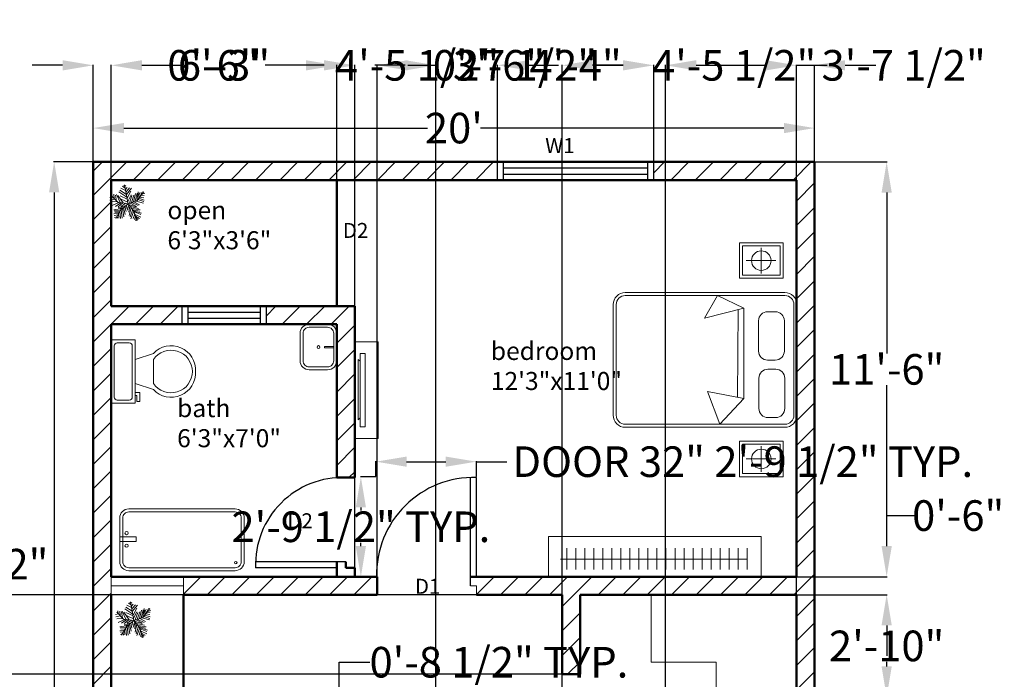
# Model space of a CAD drawing. Units: inches. Extents: x 21 to 3450, y 4 to 2137.
# Tile 14 of 14: x 3122 to 3450, y 1344 to 1563. Entities that reach past the tile are written whole.
import ezdxf

# ---------------------------------------------------------------- set-up
doc = ezdxf.new("R2010")
doc.units = ezdxf.units.IN
doc.header["$MEASUREMENT"] = 0
for name, color, linetype, lineweight in [('A-ANNO-DIMS', 2, 'Continuous', 18), ('A-ANNO-TEXT', 7, 'Continuous', 18), ('A-AREA-IDEN', 3, 'Continuous', 18), ('A-DOOR', 4, 'Continuous', 25), ('A-FLOR-FIXT', 9, 'Continuous', 18), ('A-FURN', 8, 'Continuous', 18), ('A-GLAZ', 3, 'Continuous', 25), ('A-WALL', 7, 'Continuous', 50), ('A-WALL-PATT', 8, 'Continuous', 13), ('L-PLNT', 94, 'Continuous', 13)]:
    doc.layers.add(name, color=color, linetype=linetype, lineweight=lineweight)
doc.styles.get("Standard").update_dxf_attribs({"font": 'arial.ttf'})
doc.dimstyles.get("Standard").update_dxf_attribs({"dimtxt": 10.18, "dimasz": 10.18, "dimexe": 0.18, "dimexo": 0.0625, "dimgap": 0.09, "dimtad": 0, "dimtih": 1, "dimtoh": 1, "dimdec": 0, "dimzin": 0, "dimdsep": 46, "dimlunit": 3, "dimtxsty": 'Standard', "dimcen": 0.09, "dimadec": 0, "dimazin": 0, "dimtfac": 1, "dimtdec": 0, "dimtofl": 0, "dimtmove": 0, "dimatfit": 3, "dimfxl": 1, "dimtolj": 1, "dimtzin": 0, "dimarcsym": 0})

# ---------------------------------------------------------------- blocks, each defined once
blk = doc.blocks.new('*U4')
for p, q in [((9.5, -6), (9.5, -2)), ((-10, -8.5), (-8, -8.5)), ((-10, -9.5), (-10, -8.5)), ((-7, -9.5), (-10, -9.5)), ((-8, -8.5), (-8, -8)), ((-7, -8), (-7, -9.5)), ((-4, -8), (-6, -14)), ((4, -8), (6, -14)), ((4, -14), (-4, -14))]:
    blk.add_line(p, q)
blk.add_lwpolyline([(10.5, -8), (10.5, 0), (-10.5, 0), (-10.5, -8)], close=True)
for points in [[(-9.5, -2), (-9.5, -6)], [(8.5, -1), (-8.5, -1)], [(-8.5, -7), (8.5, -7)]]:
    blk.add_lwpolyline(points)
for centre, radius, start, end in [((-8.625, -1.875), 0.8839, 81.8699, 188.1301), ((8.625, -1.875), 0.8839, 351.8699, 98.1301), ((-8.625, -6.125), 0.8839, 171.869898, 278.1301), ((8.625, -6.125), 0.8839, 261.8699, 8.1301), ((-0.4772, -19.9188), 8.0953, 133.01722, 273.38), ((0.0374, -19.8731), 7.127, 124.50543, 269.7), ((-0.0373, -19.8731), 7.127, 270.3, 55.4946), ((0.4773, -19.9188), 8.0953, 266.62, 46.9828)]:
    blk.add_arc(centre, radius, start, end)
blk = doc.blocks.new('*U6')
for p, q in [((-3.665, 19.273), (-27.574, 35.527)), ((-5.114, 28.097), (-24.676, 40.636)), ((-7.288, 39.707), (-21.778, 46.673)), ((-8.737, 47.138), (-17.069, 52.711)), ((-10.186, 53.64), (-13.084, 55.962)), ((0, 0), (-10.5, 57)), ((-9.099, 51.782), (-6.563, 55.962)), ((-7.65, 43.423), (-2.578, 49.46)), ((-5.839, 35.992), (4.667, 48.067)), ((-5.114, 27.632), (10.463, 46.673)), ((-2.941, 16.486), (8.652, 37.85)), ((16.259, 5.805), (23.142, 31.348)), ((22.055, 7.198), (27.489, 32.277)), ((27, 9), (48, 36)), ((27.127, 9.056), (31.112, 35.992)), ((31.836, 30.883), (32.561, 16.486)), ((35.096, 32.741), (37.27, 22.524)), ((38.719, 34.134), (41.979, 28.561)), ((43.791, 29.954), (51.036, 30.883)), ((44.153, 36.456), (45.239, 32.741)), ((-47.498, 19.737), (-55.83, 18.344)), ((-40.615, 13.7), (-55.105, 10.913)), ((-31.5, 4.5), (-52.5, 25.5)), ((-33.37, 6.269), (-52.207, 5.34)), ((-48.585, 21.131), (-49.309, 29.026)), ((-28.299, 3.483), (-47.86, -5.805)), ((-43.513, 28.561), (-42.427, 15.558)), ((-38.442, 26.239), (-34.819, 7.663)), ((-21.416, 3.018), (-38.079, -8.128)), ((-35.544, 28.097), (-24.314, 3.947)), ((0, 0), (-31.5, 4.5)), ((-14.533, 2.09), (-30.834, 25.31)), ((-15.982, 2.09), (-30.11, -9.521)), ((-24.314, 23.917), (-2.941, 13.7)), ((0, 0), (-22.5, -19.5)), ((-6.563, 1.161), (-21.416, -8.128)), ((-20.691, 13.7), (-1.129, 4.876)), ((-1.129, 6.734), (9.014, 26.704)), ((0, 0), (27, 9)), ((0, 0), (18, -22.5)), ((3.942, 1.625), (11.187, 24.381)), ((6.478, 1.625), (26.04, -8.592)), ((10.101, 3.483), (17.708, 26.239)), ((11.187, 3.483), (30.749, -5.805)), ((18.07, 5.805), (35.096, -3.483)), ((24.229, 7.663), (46.688, 1.625)), ((29.662, 12.307), (48.137, 6.269)), ((33.285, 16.486), (48.862, 10.913)), ((36.183, 19.737), (48.137, 17.88)), ((40.53, 25.775), (48.862, 24.846)), ((-17.431, -15.094), (-42.789, -18.809)), ((-28.299, -29.026), (-42.789, -31.348)), ((-24.314, -21.596), (-42.427, -22.06)), ((-26.849, -26.24), (-40.253, -25.775)), ((-22.5, -19.5), (-37.5, -45)), ((-15.257, -12.772), (-30.11, -12.772)), ((-25.038, -23.918), (-22.865, -45.281)), ((-20.691, -18.345), (-17.793, -44.352)), ((-6.563, -5.805), (-19.967, -9.985)), ((-17.069, -15.094), (-12.721, -40.172)), ((-13.446, -11.378), (-8.737, -32.741)), ((-9.461, -8.592), (-6.201, -23.453)), ((-4.752, -3.483), (-3.665, -14.629)), ((2.493, -3.019), (-1.491, -20.202)), ((1.769, -2.555), (24.229, -9.521)), ((5.029, -6.27), (2.131, -25.775)), ((9.014, -11.378), (3.58, -35.992)), ((14.085, -16.951), (6.478, -40.172)), ((7.565, -9.056), (32.198, -14.629)), ((18.07, -22.524), (8.289, -45.745)), ((12.274, -15.094), (36.907, -18.809)), ((16.259, -19.738), (36.183, -22.989)), ((18, -22.5), (27, -52.5)), ((18.433, -22.524), (40.53, -29.026)), ((19.157, -25.311), (38.719, -33.206)), ((-30.834, -34.135), (-42.427, -35.528)), ((-34.457, -39.708), (-40.978, -42.494)), ((-32.646, -36.921), (-31.921, -44.352)), ((-29.023, -30.884), (-27.936, -43.887)), ((20.244, -30.419), (15.897, -44.816)), ((22.78, -37.85), (19.519, -48.532)), ((21.331, -32.741), (39.081, -40.636)), ((22.78, -38.314), (34.372, -44.816)), ((24.591, -45.745), (23.142, -50.854)), ((24.591, -43.423), (30.749, -47.603)), ((26.764, -49.925), (28.213, -50.854))]:
    blk.add_line(p, q)
blk = doc.blocks.new('*D9')
at = {"layer": 'A-ANNO-DIMS', "color": 0, "lineweight": -2, "transparency": 16777216}
for p, q in [((3146.61, 1515.83), (3146.61, 1527.23)), ((3156.79, 1527.05), (3257.8, 1527.05)), ((3376.43, 1527.05), (3275.43, 1527.05)), ((3386.61, 1515.83), (3386.61, 1527.23))]:
    blk.add_line(p, q, dxfattribs=at)
at = {"layer": 'A-ANNO-DIMS', "color": 0, "transparency": 16777216}
for points in [[(3156.79, 1528.74), (3156.79, 1525.35), (3146.61, 1527.05)], [(3376.43, 1528.74), (3376.43, 1525.35), (3386.61, 1527.05)]]:
    blk.add_solid(points, dxfattribs=at)
at = {"layer": 'Defpoints', "color": 0, "transparency": 16777216}
for p in [(3386.61, 1527.05), (3146.61, 1515.77), (3386.61, 1515.77)]:
    blk.add_point(p, dxfattribs=at)
at = {"layer": 'A-ANNO-DIMS', "color": 0, "transparency": 16777216, "insert": (3266.61, 1527.05), "char_height": 10.18, "attachment_point": 5}
blk.add_mtext("\\A1;20'", dxfattribs=at)
blk = doc.blocks.new('*D10')
at = {"layer": 'A-ANNO-DIMS', "color": 0, "lineweight": -2, "transparency": 16777216}
for p, q in [((3146.55, 1515.83), (3133.43, 1515.83)), ((3133.61, 1505.65), (3133.61, 1311.09)), ((3133.61, 1105.95), (3133.61, 1300.51)), ((3329.19, 1095.77), (3133.43, 1095.77))]:
    blk.add_line(p, q, dxfattribs=at)
at = {"layer": 'A-ANNO-DIMS', "color": 0, "transparency": 16777216}
for points in [[(3131.91, 1505.65), (3135.31, 1505.65), (3133.61, 1515.83)], [(3131.91, 1105.95), (3135.31, 1105.95), (3133.61, 1095.77)]]:
    blk.add_solid(points, dxfattribs=at)
at = {"layer": 'Defpoints', "color": 0, "transparency": 16777216}
for p in [(3146.61, 1515.83), (3133.61, 1095.77), (3329.26, 1095.77)]:
    blk.add_point(p, dxfattribs=at)
at = {"layer": 'A-ANNO-DIMS', "color": 0, "transparency": 16777216, "insert": (3133.61, 1305.8), "char_height": 10.18, "attachment_point": 5}
blk.add_mtext("\\A1;35'", dxfattribs=at)
blk = doc.blocks.new('DOOR-29IN')
blk.add_line((27.01, 0), (0.01, 0))
blk.add_arc((29.01, 1), 29.02, 88.0251, 181.9749)
blk = doc.blocks.new('DOOR-32IN')
blk.add_line((33.21, 0), (33.21, 33))
blk.add_arc((32.21, 0.79), 32.22, 88.2217, 181.4078)
blk = doc.blocks.new('*D24')
at = {"layer": 'A-ANNO-DIMS', "color": 0, "lineweight": -2, "transparency": 16777216}
for p, q in [((3240.67, 1411.1), (3240.67, 1416.24)), ((3250.85, 1416.06), (3263.92, 1416.06)), ((3274.1, 1411.1), (3274.1, 1416.24)), ((3274.1, 1416.06), (3284.28, 1416.06))]:
    blk.add_line(p, q, dxfattribs=at)
at = {"layer": 'A-ANNO-DIMS', "color": 0, "transparency": 16777216}
for points in [[(3250.85, 1417.75), (3250.85, 1414.36), (3240.67, 1416.06)], [(3263.92, 1417.75), (3263.92, 1414.36), (3274.1, 1416.06)]]:
    blk.add_solid(points, dxfattribs=at)
at = {"layer": 'Defpoints', "color": 0, "transparency": 16777216}
for p in [(3274.1, 1416.06), (3240.67, 1411.04), (3274.1, 1411.04)]:
    blk.add_point(p, dxfattribs=at)
at = {"layer": 'A-ANNO-DIMS', "color": 0, "transparency": 16777216, "insert": (3362.72, 1416.06), "char_height": 10.18, "attachment_point": 5}
blk.add_mtext('\\A1;DOOR 32" 2\'-9 1/2" TYP.', dxfattribs=at)
blk = doc.blocks.new('*D25')
at = {"layer": 'A-ANNO-DIMS', "color": 0, "lineweight": -2, "transparency": 16777216}
for p, q in [((3240.61, 1411.04), (3235.48, 1411.04)), ((3235.66, 1400.86), (3235.66, 1399.76)), ((3235.66, 1387.95), (3235.66, 1389.05)), ((3240.61, 1377.77), (3235.48, 1377.77))]:
    blk.add_line(p, q, dxfattribs=at)
at = {"layer": 'A-ANNO-DIMS', "color": 0, "transparency": 16777216}
for points in [[(3233.96, 1400.86), (3237.35, 1400.86), (3235.66, 1411.04)], [(3233.96, 1387.95), (3237.35, 1387.95), (3235.66, 1377.77)]]:
    blk.add_solid(points, dxfattribs=at)
at = {"layer": 'Defpoints', "color": 0, "transparency": 16777216}
for p in [(3235.66, 1411.04), (3240.67, 1411.04), (3240.67, 1377.77)]:
    blk.add_point(p, dxfattribs=at)
at = {"layer": 'A-ANNO-DIMS', "color": 0, "transparency": 16777216, "insert": (3235.66, 1394.4), "char_height": 10.18, "attachment_point": 5}
blk.add_mtext('\\A1;2\'-9 1/2" TYP.', dxfattribs=at)
blk = doc.blocks.new('*D31')
at = {"layer": 'A-ANNO-DIMS', "color": 0, "lineweight": -2, "transparency": 16777216}
for p, q in [((3228.43, 1339.16), (3228.43, 1349.34)), ((3228.43, 1349.34), (3238.61, 1349.34)), ((3226.25, 1328.98), (3228.61, 1328.98)), ((3226.25, 1320.54), (3228.61, 1320.54)), ((3228.43, 1310.36), (3228.43, 1300.18))]:
    blk.add_line(p, q, dxfattribs=at)
at = {"layer": 'A-ANNO-DIMS', "color": 0, "transparency": 16777216}
for points in [[(3226.74, 1339.16), (3230.13, 1339.16), (3228.43, 1328.98)], [(3226.74, 1310.36), (3230.13, 1310.36), (3228.43, 1320.54)]]:
    blk.add_solid(points, dxfattribs=at)
at = {"layer": 'Defpoints', "color": 0, "transparency": 16777216}
for p in [(3226.19, 1328.98), (3228.43, 1328.98), (3226.19, 1320.54)]:
    blk.add_point(p, dxfattribs=at)
at = {"layer": 'A-ANNO-DIMS', "color": 0, "transparency": 16777216, "insert": (3281.59, 1349.34), "char_height": 10.18, "attachment_point": 5}
blk.add_mtext('\\A1;0\'-8 1/2" TYP.', dxfattribs=at)
blk = doc.blocks.new('*D32')
at = {"layer": 'A-ANNO-DIMS', "color": 0, "lineweight": -2, "transparency": 16777216}
for p, q in [((3025.36, 1314.25), (3015.18, 1314.25)), ((3035.54, 1315.23), (3035.54, 1314.07)), ((3042.48, 1315.23), (3042.48, 1314.07)), ((3052.66, 1314.25), (3062.84, 1314.25))]:
    blk.add_line(p, q, dxfattribs=at)
at = {"layer": 'A-ANNO-DIMS', "color": 0, "transparency": 16777216}
for points in [[(3025.36, 1315.95), (3025.36, 1312.56), (3035.54, 1314.25)], [(3052.66, 1315.95), (3052.66, 1312.56), (3042.48, 1314.25)]]:
    blk.add_solid(points, dxfattribs=at)
at = {"layer": 'Defpoints', "color": 0, "transparency": 16777216}
for p in [(3035.54, 1315.29), (3042.48, 1315.29), (3042.48, 1314.25)]:
    blk.add_point(p, dxfattribs=at)
at = {"layer": 'A-ANNO-DIMS', "color": 0, "transparency": 16777216, "insert": (3152.02, 1314.25), "char_height": 10.18, "attachment_point": 5}
blk.add_mtext('\\A1;STOVE BURNER 0\'-7" TYP.', dxfattribs=at)
blk = doc.blocks.new('*D123')
at = {"layer": 'A-ANNO-DIMS', "color": 0, "lineweight": -2, "transparency": 16777216}
for p, q in [((3136.43, 1547.93), (3126.25, 1547.93)), ((3146.61, 1515.83), (3146.61, 1548.11)), ((3152.61, 1509.83), (3152.61, 1548.11)), ((3162.79, 1547.93), (3172.97, 1547.93))]:
    blk.add_line(p, q, dxfattribs=at)
at = {"layer": 'A-ANNO-DIMS', "color": 0, "transparency": 16777216}
for points in [[(3136.43, 1549.63), (3136.43, 1546.23), (3146.61, 1547.93)], [(3162.79, 1549.63), (3162.79, 1546.23), (3152.61, 1547.93)]]:
    blk.add_solid(points, dxfattribs=at)
at = {"layer": 'Defpoints', "color": 0, "transparency": 16777216}
for p in [(3152.61, 1547.93), (3146.61, 1515.77), (3152.61, 1509.77)]:
    blk.add_point(p, dxfattribs=at)
at = {"layer": 'A-ANNO-DIMS', "color": 0, "transparency": 16777216, "insert": (3186.59, 1547.93), "char_height": 10.18, "attachment_point": 5}
blk.add_mtext('\\A1;0\'-6"', dxfattribs=at)
blk = doc.blocks.new('*D124')
at = {"layer": 'A-ANNO-DIMS', "color": 0, "lineweight": -2, "transparency": 16777216}
for p, q in [((3152.61, 1509.83), (3152.61, 1548.11)), ((3162.79, 1547.93), (3176.46, 1547.93)), ((3217.43, 1547.93), (3203.76, 1547.93)), ((3227.61, 1509.83), (3227.61, 1548.11))]:
    blk.add_line(p, q, dxfattribs=at)
at = {"layer": 'A-ANNO-DIMS', "color": 0, "transparency": 16777216}
for points in [[(3162.79, 1549.63), (3162.79, 1546.23), (3152.61, 1547.93)], [(3217.43, 1549.63), (3217.43, 1546.23), (3227.61, 1547.93)]]:
    blk.add_solid(points, dxfattribs=at)
at = {"layer": 'Defpoints', "color": 0, "transparency": 16777216}
for p in [(3227.61, 1547.93), (3152.61, 1509.77), (3227.61, 1509.77)]:
    blk.add_point(p, dxfattribs=at)
at = {"layer": 'A-ANNO-DIMS', "color": 0, "transparency": 16777216, "insert": (3190.11, 1547.93), "char_height": 10.18, "attachment_point": 5}
blk.add_mtext('\\A1;6\'-3"', dxfattribs=at)
blk = doc.blocks.new('*D125')
at = {"layer": 'A-ANNO-DIMS', "color": 0, "lineweight": -2, "transparency": 16777216}
for p, q in [((3217.43, 1547.93), (3207.25, 1547.93)), ((3227.61, 1509.83), (3227.61, 1548.11)), ((3281.11, 1515.83), (3281.11, 1548.11)), ((3291.29, 1547.93), (3301.47, 1547.93))]:
    blk.add_line(p, q, dxfattribs=at)
at = {"layer": 'A-ANNO-DIMS', "color": 0, "transparency": 16777216}
for points in [[(3217.43, 1549.63), (3217.43, 1546.23), (3227.61, 1547.93)], [(3291.29, 1549.63), (3291.29, 1546.23), (3281.11, 1547.93)]]:
    blk.add_solid(points, dxfattribs=at)
at = {"layer": 'Defpoints', "color": 0, "transparency": 16777216}
for p in [(3281.11, 1547.93), (3281.11, 1515.77), (3227.61, 1509.77)]:
    blk.add_point(p, dxfattribs=at)
at = {"layer": 'A-ANNO-DIMS', "color": 0, "transparency": 16777216, "insert": (3254.36, 1547.93), "char_height": 10.18, "attachment_point": 5}
blk.add_mtext('\\A1;4\'-5 1/2"', dxfattribs=at)
blk = doc.blocks.new('*D126')
at = {"layer": 'A-ANNO-DIMS', "color": 0, "lineweight": -2, "transparency": 16777216}
for p, q in [((3281.11, 1515.83), (3281.11, 1548.11)), ((3291.29, 1547.93), (3293.29, 1547.93)), ((3322.93, 1547.93), (3320.94, 1547.93)), ((3333.11, 1515.83), (3333.11, 1548.11))]:
    blk.add_line(p, q, dxfattribs=at)
at = {"layer": 'A-ANNO-DIMS', "color": 0, "transparency": 16777216}
for points in [[(3291.29, 1549.63), (3291.29, 1546.23), (3281.11, 1547.93)], [(3322.93, 1549.63), (3322.93, 1546.23), (3333.11, 1547.93)]]:
    blk.add_solid(points, dxfattribs=at)
at = {"layer": 'Defpoints', "color": 0, "transparency": 16777216}
for p in [(3333.11, 1547.93), (3281.11, 1515.77), (3333.11, 1515.77)]:
    blk.add_point(p, dxfattribs=at)
at = {"layer": 'A-ANNO-DIMS', "color": 0, "transparency": 16777216, "insert": (3307.11, 1547.93), "char_height": 10.18, "attachment_point": 5}
blk.add_mtext('\\A1;4\'-4"', dxfattribs=at)
blk = doc.blocks.new('*D127')
at = {"layer": 'A-ANNO-DIMS', "color": 0, "lineweight": -2, "transparency": 16777216}
for p, q in [((3322.93, 1547.93), (3312.75, 1547.93)), ((3333.11, 1515.83), (3333.11, 1548.11)), ((3386.61, 1515.83), (3386.61, 1548.11)), ((3396.79, 1547.93), (3406.97, 1547.93))]:
    blk.add_line(p, q, dxfattribs=at)
at = {"layer": 'A-ANNO-DIMS', "color": 0, "transparency": 16777216}
for points in [[(3322.93, 1549.63), (3322.93, 1546.23), (3333.11, 1547.93)], [(3396.79, 1549.63), (3396.79, 1546.23), (3386.61, 1547.93)]]:
    blk.add_solid(points, dxfattribs=at)
at = {"layer": 'Defpoints', "color": 0, "transparency": 16777216}
for p in [(3386.61, 1547.93), (3333.11, 1515.77), (3386.61, 1515.77)]:
    blk.add_point(p, dxfattribs=at)
at = {"layer": 'A-ANNO-DIMS', "color": 0, "transparency": 16777216, "insert": (3359.86, 1547.93), "char_height": 10.18, "attachment_point": 5}
blk.add_mtext('\\A1;4\'-5 1/2"', dxfattribs=at)
blk = doc.blocks.new('*D138')
at = {"layer": 'A-ANNO-DIMS', "color": 0, "lineweight": -2, "transparency": 16777216}
for p, q in [((3380.67, 1371.77), (3410.79, 1371.77)), ((3410.61, 1361.59), (3410.61, 1360.05)), ((3410.61, 1347.95), (3410.61, 1349.48)), ((3386.67, 1337.77), (3410.79, 1337.77))]:
    blk.add_line(p, q, dxfattribs=at)
at = {"layer": 'A-ANNO-DIMS', "color": 0, "transparency": 16777216}
for points in [[(3408.91, 1361.59), (3412.31, 1361.59), (3410.61, 1371.77)], [(3408.91, 1347.95), (3412.31, 1347.95), (3410.61, 1337.77)]]:
    blk.add_solid(points, dxfattribs=at)
at = {"layer": 'Defpoints', "color": 0, "transparency": 16777216}
for p in [(3380.61, 1371.77), (3410.61, 1371.77), (3386.61, 1337.77)]:
    blk.add_point(p, dxfattribs=at)
at = {"layer": 'A-ANNO-DIMS', "color": 0, "transparency": 16777216, "insert": (3410.61, 1354.77), "char_height": 10.18, "attachment_point": 5}
blk.add_mtext('\\A1;2\'-10"', dxfattribs=at)
blk = doc.blocks.new('*D139')
at = {"layer": 'A-ANNO-DIMS', "color": 0, "lineweight": -2, "transparency": 16777216}
for p, q in [((3410.61, 1387.95), (3410.61, 1398.13)), ((3410.61, 1398.13), (3420.79, 1398.13)), ((3380.67, 1377.77), (3410.79, 1377.77)), ((3380.67, 1371.77), (3410.79, 1371.77)), ((3410.61, 1361.59), (3410.61, 1351.41))]:
    blk.add_line(p, q, dxfattribs=at)
at = {"layer": 'A-ANNO-DIMS', "color": 0, "transparency": 16777216}
for points in [[(3408.91, 1387.95), (3412.31, 1387.95), (3410.61, 1377.77)], [(3408.91, 1361.59), (3412.31, 1361.59), (3410.61, 1371.77)]]:
    blk.add_solid(points, dxfattribs=at)
at = {"layer": 'Defpoints', "color": 0, "transparency": 16777216}
for p in [(3380.61, 1377.77), (3410.61, 1377.77), (3380.61, 1371.77)]:
    blk.add_point(p, dxfattribs=at)
at = {"layer": 'A-ANNO-DIMS', "color": 0, "transparency": 16777216, "insert": (3434.41, 1398.13), "char_height": 10.18, "attachment_point": 5}
blk.add_mtext('\\A1;0\'-6"', dxfattribs=at)
blk = doc.blocks.new('*D140')
at = {"layer": 'A-ANNO-DIMS', "color": 0, "lineweight": -2, "transparency": 16777216}
for p, q in [((3386.67, 1515.77), (3410.79, 1515.77)), ((3410.61, 1505.59), (3410.61, 1452.05)), ((3410.61, 1387.95), (3410.61, 1441.48)), ((3380.67, 1377.77), (3410.79, 1377.77))]:
    blk.add_line(p, q, dxfattribs=at)
at = {"layer": 'A-ANNO-DIMS', "color": 0, "transparency": 16777216}
for points in [[(3408.91, 1505.59), (3412.31, 1505.59), (3410.61, 1515.77)], [(3408.91, 1387.95), (3412.31, 1387.95), (3410.61, 1377.77)]]:
    blk.add_solid(points, dxfattribs=at)
at = {"layer": 'Defpoints', "color": 0, "transparency": 16777216}
for p in [(3386.61, 1515.77), (3410.61, 1515.77), (3380.61, 1377.77)]:
    blk.add_point(p, dxfattribs=at)
at = {"layer": 'A-ANNO-DIMS', "color": 0, "transparency": 16777216, "insert": (3410.61, 1446.77), "char_height": 10.18, "attachment_point": 5}
blk.add_mtext('\\A1;11\'-6"', dxfattribs=at)
blk = doc.blocks.new('*D143')
at = {"layer": 'A-ANNO-DIMS', "color": 0, "lineweight": -2, "transparency": 16777216}
for p, q in [((3223.43, 1547.93), (3213.25, 1547.93)), ((3233.61, 1377.83), (3233.61, 1548.11)), ((3241.1, 1377.83), (3241.1, 1548.11)), ((3251.28, 1547.93), (3261.46, 1547.93))]:
    blk.add_line(p, q, dxfattribs=at)
at = {"layer": 'A-ANNO-DIMS', "color": 0, "transparency": 16777216}
for points in [[(3223.43, 1549.63), (3223.43, 1546.23), (3233.61, 1547.93)], [(3251.28, 1549.63), (3251.28, 1546.23), (3241.1, 1547.93)]]:
    blk.add_solid(points, dxfattribs=at)
at = {"layer": 'Defpoints', "color": 0, "transparency": 16777216}
for p in [(3241.1, 1547.93), (3233.61, 1377.77), (3241.1, 1377.77)]:
    blk.add_point(p, dxfattribs=at)
at = {"layer": 'A-ANNO-DIMS', "color": 0, "transparency": 16777216, "insert": (3286.94, 1547.93), "char_height": 10.18, "attachment_point": 5}
blk.add_mtext('\\A1;0\'-7 1/2"', dxfattribs=at)
blk = doc.blocks.new('*D145')
at = {"layer": 'A-ANNO-DIMS', "color": 0, "lineweight": -2, "transparency": 16777216}
for p, q in [((3250.43, 1547.93), (3240.25, 1547.93)), ((3260.61, 1251.83), (3260.61, 1548.11)), ((3302.61, 1251.83), (3302.61, 1548.11)), ((3312.79, 1547.93), (3322.97, 1547.93))]:
    blk.add_line(p, q, dxfattribs=at)
at = {"layer": 'A-ANNO-DIMS', "color": 0, "transparency": 16777216}
for points in [[(3250.43, 1549.63), (3250.43, 1546.23), (3260.61, 1547.93)], [(3312.79, 1549.63), (3312.79, 1546.23), (3302.61, 1547.93)]]:
    blk.add_solid(points, dxfattribs=at)
at = {"layer": 'Defpoints', "color": 0, "transparency": 16777216}
for p in [(3302.61, 1547.93), (3260.61, 1251.77), (3302.61, 1251.77)]:
    blk.add_point(p, dxfattribs=at)
at = {"layer": 'A-ANNO-DIMS', "color": 0, "transparency": 16777216, "insert": (3281.61, 1547.93), "char_height": 10.18, "attachment_point": 5}
blk.add_mtext('\\A1;3\'-6"', dxfattribs=at)
blk = doc.blocks.new('*D146')
at = {"layer": 'A-ANNO-DIMS', "color": 0, "lineweight": -2, "transparency": 16777216}
for p, q in [((3068.61, 1371.77), (3068.61, 1381.95)), ((3068.61, 1381.95), (3078.79, 1381.95)), ((3302.55, 1371.77), (3068.43, 1371.77)), ((3068.61, 1355.5), (3068.61, 1361.59)), ((3302.55, 1345.32), (3068.43, 1345.32))]:
    blk.add_line(p, q, dxfattribs=at)
at = {"layer": 'A-ANNO-DIMS', "color": 0, "transparency": 16777216}
for points in [[(3066.91, 1361.59), (3070.31, 1361.59), (3068.61, 1371.77)], [(3066.91, 1355.5), (3070.31, 1355.5), (3068.61, 1345.32)]]:
    blk.add_solid(points, dxfattribs=at)
at = {"layer": 'Defpoints', "color": 0, "transparency": 16777216}
for p in [(3068.61, 1371.77), (3302.61, 1371.77), (3302.61, 1345.32)]:
    blk.add_point(p, dxfattribs=at)
at = {"layer": 'A-ANNO-DIMS', "color": 0, "transparency": 16777216, "insert": (3104.36, 1381.95), "char_height": 10.18, "attachment_point": 5}
blk.add_mtext('\\A1;2\'-2 1/2"', dxfattribs=at)
blk = doc.blocks.new('*D148')
at = {"layer": 'A-ANNO-DIMS', "color": 0, "lineweight": -2, "transparency": 16777216}
for p, q in [((3337.06, 1101.83), (3337.06, 1548.11)), ((3347.24, 1547.93), (3370.43, 1547.93)), ((3380.61, 1101.83), (3380.61, 1548.11)), ((3380.61, 1547.93), (3390.79, 1547.93))]:
    blk.add_line(p, q, dxfattribs=at)
at = {"layer": 'A-ANNO-DIMS', "color": 0, "transparency": 16777216}
for points in [[(3347.24, 1549.63), (3347.24, 1546.23), (3337.06, 1547.93)], [(3370.43, 1549.63), (3370.43, 1546.23), (3380.61, 1547.93)]]:
    blk.add_solid(points, dxfattribs=at)
at = {"layer": 'Defpoints', "color": 0, "transparency": 16777216}
for p in [(3380.61, 1547.93), (3337.06, 1101.77), (3380.61, 1101.77)]:
    blk.add_point(p, dxfattribs=at)
at = {"layer": 'A-ANNO-DIMS', "color": 0, "transparency": 16777216, "insert": (3416.27, 1547.93), "char_height": 10.18, "attachment_point": 5}
blk.add_mtext('\\A1;3\'-7 1/2"', dxfattribs=at)

msp = doc.modelspace()

# ---------------------------------------------------------------- hatches: boundary and pattern name
at = {"layer": 'A-WALL-PATT'}
h = msp.add_hatch(dxfattribs=at)
h.set_pattern_fill('ANSI31', color=256, scale=46)
h.set_pattern_definition([(45, (297.6833, 160.0466), (-4.065864, 4.065864), [])])
h.paths.add_polyline_path([(3281.11, 1515.77), (3146.61, 1515.77), (3146.61, 1199.77), (3152.61, 1199.77), (3152.61, 1245.77), (3152.61, 1251.77), (3152.61, 1371.77), (3152.61, 1377.77), (3152.61, 1461.77), (3176.11, 1461.77), (3176.11, 1467.77), (3152.61, 1467.77), (3152.61, 1509.77), (3227.61, 1509.77), (3233.61, 1509.77), (3281.11, 1509.77)])
h.paths.add_polyline_path([(3386.61, 1515.77), (3333.11, 1515.77), (3333.11, 1509.77), (3380.61, 1509.77), (3380.61, 1469.33, -0.065004), (3380.75, 1468.31), (3380.75, 1431.5, -0.065004), (3380.61, 1430.47), (3380.61, 1377.77), (3272.1, 1377.77), (3272.1, 1374.77), (3274.1, 1374.77), (3274.1, 1371.77), (3302.61, 1371.77), (3302.61, 1345.32), (3308.61, 1345.32), (3308.61, 1371.77), (3380.61, 1371.77), (3380.61, 1337.77), (3386.61, 1337.77)])
h.paths.add_polyline_path([(3215.61, 1248.77), (3215.61, 1251.77), (3182.61, 1251.77), (3182.61, 1333.19), (3176.61, 1333.19), (3176.61, 1251.77), (3176.61, 1245.77), (3215.61, 1245.77), (3215.61, 1246.77, -0.014283)], flags=17)
h.paths.add_polyline_path([(3177.61, 1101.77), (3152.61, 1101.77), (3152.61, 1147.77), (3146.61, 1147.77), (3146.61, 1095.77), (3177.61, 1095.77)])
h.paths.add_polyline_path([(3241.1, 1377.77), (3233.61, 1377.77), (3227.61, 1377.77), (3176.61, 1377.77), (3176.61, 1371.77), (3182.61, 1371.77), (3233.61, 1371.77), (3241.1, 1371.77)], flags=17)
h.paths.add_polyline_path([(3233.61, 1467.77), (3227.61, 1467.77), (3204.11, 1467.77), (3204.11, 1461.77), (3227.61, 1461.77), (3227.61, 1410.77), (3228.61, 1410.77, -0.017236), (3230.61, 1410.77), (3233.61, 1410.77), (3233.61, 1461.77)], flags=17)

# ---------------------------------------------------------------- linework, layer by layer
at = {"layer": 'A-DOOR'}
for p, q in [((3272.1, 1374.77), (3272.1, 1410.77)), ((3230.61, 1382.77), (3200.61, 1382.77))]:
    msp.add_line(p, q, dxfattribs=at)
at = {"layer": 'A-FLOR-FIXT'}
for p, q in [((3152.61, 1377.77), (3152.61, 1371.77)), ((3176.61, 1371.77), (3176.61, 1377.77)), ((3176.61, 1374.77), (3152.61, 1374.77)), ((3152.61, 1371.77), (3176.61, 1371.77)), ((3353.85, 1251.77), (3353.85, 1349.33))]:
    msp.add_line(p, q, dxfattribs=at)
for points in [[(3158.42, 1379.79, -0.414214), (3155.42, 1382.79), (3155.42, 1397.33, -0.414214), (3158.42, 1400.33), (3193.83, 1400.33, -0.414214), (3196.83, 1397.33), (3196.83, 1382.79, -0.414214), (3193.83, 1379.79)], [(3158.42, 1380.79, -0.414214), (3156.42, 1382.79), (3156.42, 1397.33, -0.414214), (3158.42, 1399.33), (3193.83, 1399.33, -0.414214), (3195.83, 1397.33), (3195.83, 1382.79, -0.414214), (3193.83, 1380.79)]]:
    msp.add_lwpolyline(points, format="xyb", close=True, dxfattribs=at)
msp.add_lwpolyline([(3155.42, 1391.07), (3155.42, 1391.07), (3160.86, 1391.07), (3160.86, 1391.07), (3160.86, 1389.48), (3160.86, 1389.48), (3155.42, 1389.48), (3155.42, 1389.48)], close=True, dxfattribs=at)
for centre, radius in [((3157.68, 1392.28), 0.546), ((3157.68, 1388.11), 0.546), ((3194.05, 1382.48), 0.395)]:
    msp.add_circle(centre, radius, dxfattribs=at)
at = {"layer": 'A-FURN'}
for p, q in [((3368.89, 1487.24), (3368.89, 1478.71)), ((3363.81, 1482.96), (3373.75, 1482.96)), ((3354.33, 1471.31), (3350.02, 1463.83)), ((3363.05, 1467.12), (3354.33, 1471.31)), ((3350.02, 1463.83), (3363.05, 1467.12)), ((3361.25, 1466.67), (3361.03, 1437.43)), ((3363.05, 1467.12), (3363.05, 1437.03)), ((3235.44, 1449.47), (3234.76, 1450.1)), ((3234.76, 1450.1), (3234.76, 1430.02)), ((3355.08, 1428.5), (3351.01, 1439.4)), ((3351.01, 1439.4), (3363.05, 1437.03)), ((3363.05, 1437.03), (3355.08, 1428.5)), ((3234.76, 1430.02), (3235.44, 1430.69)), ((3368.89, 1421.24), (3368.89, 1412.7)), ((3363.81, 1416.96), (3373.75, 1416.96)), ((3304.18, 1387.26), (3304.18, 1380.17)), ((3307.18, 1387.26), (3307.18, 1380.17)), ((3310.18, 1387.26), (3310.18, 1380.17)), ((3313.18, 1387.26), (3313.18, 1380.17)), ((3316.18, 1387.26), (3316.18, 1380.17)), ((3319.18, 1387.26), (3319.18, 1380.17)), ((3322.18, 1387.26), (3322.18, 1380.17)), ((3325.18, 1387.26), (3325.18, 1380.17)), ((3328.18, 1387.26), (3328.18, 1380.17)), ((3331.18, 1387.26), (3331.18, 1380.17)), ((3334.18, 1387.26), (3334.18, 1380.17)), ((3337.18, 1387.26), (3337.18, 1380.17)), ((3340.18, 1387.26), (3340.18, 1380.17)), ((3343.18, 1387.26), (3343.18, 1380.17)), ((3346.18, 1387.26), (3346.18, 1380.17)), ((3349.18, 1387.26), (3349.18, 1380.17)), ((3352.18, 1387.26), (3352.18, 1380.17)), ((3355.18, 1387.26), (3355.18, 1380.17)), ((3358.18, 1387.26), (3358.18, 1380.17)), ((3361.18, 1387.26), (3361.18, 1380.17)), ((3364.18, 1387.26), (3364.18, 1380.17)), ((3302.1, 1383.65), (3364.16, 1383.65)), ((3272.1, 1374.77), (3274.1, 1374.77)), ((3274.1, 1374.77), (3274.1, 1371.77)), ((3332.24, 1349.33), (3332.24, 1371.77)), ((3353.85, 1349.33), (3332.24, 1349.33))]:
    msp.add_line(p, q, dxfattribs=at)
for points in [[(3361.59, 1488.85), (3361.59, 1488.85), (3376.2, 1488.85), (3376.2, 1488.85), (3376.2, 1477.07), (3376.2, 1477.07), (3361.59, 1477.07), (3361.59, 1477.07)], [(3362.59, 1487.85), (3375.2, 1487.85), (3375.2, 1478.07), (3362.59, 1478.07)], [(3233.61, 1455.89), (3233.61, 1455.89), (3241.44, 1455.89), (3241.44, 1455.89), (3241.44, 1423.77), (3241.44, 1423.77), (3233.61, 1423.77), (3233.61, 1423.77)], [(3226.61, 1454.43), (3226.61, 1454.43), (3223.61, 1454.43), (3223.61, 1454.43), (3223.61, 1453.91), (3223.61, 1453.91), (3226.61, 1453.91), (3226.61, 1453.91)], [(3235.44, 1452.07), (3235.44, 1452.07), (3237.05, 1452.07), (3237.05, 1452.07), (3237.05, 1427.6), (3237.05, 1427.6), (3235.44, 1427.6), (3235.44, 1427.6)], [(3361.59, 1422.85), (3361.59, 1422.85), (3376.2, 1422.85), (3376.2, 1422.85), (3376.2, 1411.07), (3376.2, 1411.07), (3361.59, 1411.07), (3361.59, 1411.07)], [(3362.59, 1421.85), (3375.2, 1421.85), (3375.2, 1412.07), (3362.59, 1412.07)], [(3368.89, 1377.77), (3368.89, 1377.77), (3298.14, 1377.77), (3298.14, 1377.77), (3298.14, 1391.19), (3298.14, 1391.19), (3368.89, 1391.19), (3368.89, 1391.19)]]:
    msp.add_lwpolyline(points, close=True, dxfattribs=at)
for points in [[(3380.75, 1468.31, 0.414214), (3376.75, 1472.31), (3323.62, 1472.31, 0.414214), (3319.62, 1468.31), (3319.62, 1431.5, 0.414214), (3323.62, 1427.5), (3376.75, 1427.5, 0.414214), (3380.75, 1431.5)], [(3379.75, 1468.31, 0.414214), (3376.75, 1471.31), (3323.62, 1471.31, 0.414214), (3320.62, 1468.31), (3320.62, 1431.5, 0.414214), (3323.62, 1428.5), (3376.75, 1428.5, 0.414214), (3379.75, 1431.5)], [(3367.97, 1462.94, -0.414214), (3370.97, 1465.94), (3373.56, 1465.94, -0.414214), (3376.56, 1462.94), (3376.56, 1452.87, -0.414214), (3373.56, 1449.87), (3370.97, 1449.87, -0.414214), (3367.97, 1452.87)], [(3227.61, 1458.77, 0.414214), (3224.61, 1461.77), (3218.45, 1461.77, 0.414214), (3215.45, 1458.77), (3215.45, 1449.62, 0.414214), (3218.45, 1446.62), (3224.61, 1446.62, 0.414214), (3227.61, 1449.62)], [(3226.61, 1458.77, 0.414214), (3224.61, 1460.77), (3218.45, 1460.77, 0.414214), (3216.45, 1458.77), (3216.45, 1449.62, 0.414214), (3218.45, 1447.62), (3224.61, 1447.62, 0.414214), (3226.61, 1449.62)], [(3368.12, 1443.8, -0.414214), (3371.12, 1446.8), (3373.71, 1446.8, -0.414214), (3376.71, 1443.8), (3376.71, 1433.74, -0.414214), (3373.71, 1430.74), (3371.12, 1430.74, -0.414214), (3368.12, 1433.74)]]:
    msp.add_lwpolyline(points, format="xyb", close=True, dxfattribs=at)
for centre, radius in [((3368.89, 1482.96), 3.25), ((3221.53, 1454.2), 0.458), ((3368.89, 1416.96), 3.25)]:
    msp.add_circle(centre, radius, dxfattribs=at)
at = {"layer": 'A-GLAZ'}
for p, q in [((3281.11, 1509.77), (3281.11, 1515.77)), ((3283.11, 1509.77), (3283.11, 1515.77)), ((3283.11, 1513.77), (3331.11, 1513.77)), ((3331.11, 1509.77), (3331.11, 1515.77)), ((3333.11, 1509.77), (3333.11, 1515.77)), ((3283.11, 1511.77), (3331.11, 1511.77)), ((3176.11, 1467.77), (3176.11, 1461.77)), ((3178.11, 1467.77), (3178.11, 1461.77)), ((3202.11, 1467.77), (3202.11, 1461.77)), ((3204.11, 1467.77), (3204.11, 1461.77)), ((3178.11, 1465.77), (3202.11, 1465.77)), ((3178.11, 1463.77), (3202.11, 1463.77))]:
    msp.add_line(p, q, dxfattribs=at)
at = {"layer": 'A-WALL'}
for p, q in [((3146.61, 1095.77), (3146.61, 1515.77)), ((3146.61, 1515.77), (3386.61, 1515.77)), ((3386.61, 1515.77), (3386.61, 1095.77)), ((3152.61, 1467.77), (3152.61, 1509.77)), ((3152.61, 1509.77), (3227.61, 1509.77)), ((3227.61, 1509.77), (3233.61, 1509.77)), ((3227.61, 1467.77), (3227.61, 1509.77)), ((3233.61, 1509.77), (3380.61, 1509.77)), ((3380.61, 1509.77), (3380.61, 1377.77)), ((3152.61, 1467.77), (3227.61, 1467.77)), ((3227.61, 1467.77), (3233.61, 1467.77)), ((3233.61, 1461.77), (3233.61, 1467.77)), ((3152.61, 1377.77), (3152.61, 1461.77)), ((3152.61, 1461.77), (3227.61, 1461.77)), ((3227.61, 1410.71), (3227.61, 1461.77)), ((3233.61, 1410.77), (3233.61, 1461.77)), ((3227.61, 1410.77), (3233.61, 1410.77)), ((3227.61, 1377.77), (3227.61, 1382.77)), ((3230.61, 1382.77), (3230.61, 1380.77)), ((3230.61, 1380.77), (3233.61, 1380.77)), ((3233.61, 1377.77), (3233.61, 1380.77)), ((3152.61, 1377.77), (3227.61, 1377.77)), ((3227.61, 1377.77), (3233.61, 1377.77)), ((3233.61, 1377.77), (3241.1, 1377.77)), ((3241.1, 1377.77), (3241.1, 1371.77)), ((3272.1, 1377.77), (3380.61, 1377.77)), ((3152.61, 1251.77), (3152.61, 1371.77)), ((3176.61, 1371.77), (3176.61, 1251.77)), ((3182.61, 1371.77), (3176.61, 1371.77)), ((3182.61, 1371.77), (3233.61, 1371.77)), ((3233.61, 1371.77), (3241.1, 1371.77)), ((3274.1, 1371.77), (3302.61, 1371.77)), ((3302.61, 1371.77), (3302.61, 1345.32)), ((3308.61, 1371.77), (3380.61, 1371.77)), ((3308.61, 1371.77), (3308.61, 1345.32)), ((3380.61, 1371.77), (3380.61, 1251.77)), ((3302.61, 1345.32), (3308.61, 1345.32))]:
    msp.add_line(p, q, dxfattribs=at)

# ---------------------------------------------------------------- block references
at = {"layer": 'A-DOOR'}
for name, p in [('DOOR-29IN', (3200.6, 1380.77)), ('DOOR-32IN', (3240.89, 1377.77))]:
    msp.add_blockref(name, p, dxfattribs=at)
at = {"layer": 'A-FLOR-FIXT', "rotation": 90}
msp.add_blockref('*U4', (3152.61, 1446.06), dxfattribs=at)
at = {"layer": 'L-PLNT', "xscale": 0.1095009231923873, "yscale": 0.1095009231923873, "zscale": 0.1095009231923873}
for p in [(3158.19, 1501.9), (3160.17, 1363.22)]:
    msp.add_blockref('*U6', p, dxfattribs=at)

# ---------------------------------------------------------------- texts
at = {"layer": 'A-ANNO-TEXT', "char_height": 5, "attachment_point": 1}
for s, insert in [('W1', (3297, 1523.71)), ('D2', (3229.66, 1495.49)), ('D2', (3211.2, 1398.89)), ('D1', (3253.64, 1377.1))]:
    msp.add_mtext_dynamic_manual_height_columns(s, width=14.628, gutter_width=1, heights=[0], dxfattribs=dict(at, insert=insert))
at = {"layer": 'A-AREA-IDEN', "char_height": 6, "attachment_point": 1}
for s, insert in [('open\\P6\'3"x3\'6"', (3171.29, 1502.73)), ('bedroom\\P12\'3"x11\'0"', (3278.91, 1455.9)), ('bath\\P6\'3"x7\'0"', (3174.52, 1436.87))]:
    msp.add_mtext_dynamic_manual_height_columns(s, width=84.0083, gutter_width=1, heights=[0], dxfattribs=dict(at, insert=insert))

# ---------------------------------------------------------------- dimensions: what is measured, and where the dimension line sits
at = {"layer": 'A-ANNO-DIMS'}
for base, p1, p2, override, picture, middle in [((3281.11, 1547.93), (3227.61, 1509.77), (3281.11, 1515.77), {"dimdec": 1, "dimlfac": 1, "dimrnd": 0, "dimzin": 1, "dimdsep": 46, "dimlunit": 4, "dimfrac": 2}, '*D125', (3254.36, 1547.93)), ((3241.1, 1547.93), (3233.61, 1377.77), (3241.1, 1377.77), {"dimdec": 1, "dimlfac": 1, "dimrnd": 0, "dimzin": 1, "dimdsep": 46, "dimlunit": 4, "dimfrac": 2}, '*D143', (3286.94, 1547.93)), ((3386.61, 1547.93), (3333.11, 1515.77), (3386.61, 1515.77), {"dimdec": 1, "dimlfac": 1, "dimrnd": 0, "dimzin": 1, "dimdsep": 46, "dimlunit": 4, "dimfrac": 2}, '*D127', (3359.86, 1547.93)), ((3380.611, 1547.9292), (3337.0593, 1101.7664), (3380.611, 1101.7664), {"dimdec": 1, "dimlfac": 1, "dimrnd": 0, "dimzin": 1, "dimdsep": 46, "dimlunit": 4, "dimfrac": 2}, '*D148', (3416.2685, 1547.9292)), ((3152.61, 1547.93), (3146.61, 1515.77), (3152.61, 1509.77), {"dimdec": 1, "dimlfac": 1, "dimrnd": 0, "dimzin": 1, "dimdsep": 46, "dimlunit": 4, "dimfrac": 2}, '*D123', (3186.59, 1547.93)), ((3227.61, 1547.93), (3152.61, 1509.77), (3227.61, 1509.77), {"dimdec": 1, "dimlfac": 1, "dimrnd": 0, "dimzin": 1, "dimdsep": 46, "dimlunit": 4, "dimfrac": 2}, '*D124', (3190.11, 1547.93)), ((3302.61, 1547.93), (3260.61, 1251.77), (3302.61, 1251.77), {"dimdec": 1, "dimlfac": 1, "dimrnd": 0, "dimzin": 1, "dimdsep": 46, "dimlunit": 4, "dimfrac": 2}, '*D145', (3281.61, 1547.93)), ((3333.11, 1547.93), (3281.11, 1515.77), (3333.11, 1515.77), {"dimdec": 1, "dimlfac": 1, "dimrnd": 0, "dimzin": 1, "dimdsep": 46, "dimlunit": 4, "dimfrac": 2}, '*D126', (3307.11, 1547.93)), ((3386.61, 1527.05), (3146.61, 1515.77), (3386.61, 1515.77), {"dimclrd": 0, "dimclre": 0, "dimclrt": 0}, '*D9', (3266.61, 1527.05))]:
    dim = msp.add_linear_dim(base=base, p1=p1, p2=p2, dimstyle='Standard', override=override, dxfattribs=at)
    dim.commit()
    dim.dimension.update_dxf_attribs({"geometry": picture, "text_midpoint": middle})
for base, p1, p2, override, picture, middle in [((3133.61, 1095.77), (3146.61, 1515.83), (3329.26, 1095.77), {"dimclrd": 0, "dimclre": 0, "dimclrt": 0}, '*D10', (3133.61, 1305.8)), ((3410.61, 1515.77), (3380.61, 1377.77), (3386.61, 1515.77), {"dimdec": 1, "dimlfac": 1, "dimrnd": 0, "dimzin": 1, "dimdsep": 46, "dimlunit": 4, "dimfrac": 2}, '*D140', (3410.61, 1446.77)), ((3410.61, 1377.77), (3380.61, 1371.77), (3380.61, 1377.77), {"dimdec": 1, "dimlfac": 1, "dimrnd": 0, "dimzin": 1, "dimdsep": 46, "dimlunit": 4, "dimfrac": 2}, '*D139', (3434.41, 1398.13)), ((3068.611, 1371.7664), (3302.611, 1345.3178), (3302.611, 1371.7664), {"dimdec": 1, "dimlfac": 1, "dimrnd": 0, "dimzin": 1, "dimdsep": 46, "dimlunit": 4, "dimfrac": 2}, '*D146', (3104.3587, 1381.9464)), ((3410.61, 1371.77), (3386.61, 1337.77), (3380.61, 1371.77), {"dimdec": 1, "dimlfac": 1, "dimrnd": 0, "dimzin": 1, "dimdsep": 46, "dimlunit": 4, "dimfrac": 2}, '*D138', (3410.61, 1354.77))]:
    dim = msp.add_linear_dim(base=base, p1=p1, p2=p2, angle=90, dimstyle='Standard', override=override, dxfattribs=at)
    dim.commit()
    dim.dimension.update_dxf_attribs({"geometry": picture, "text_midpoint": middle})
for base, p1, p2, text, picture, middle in [((3274.1, 1416.06), (3240.67, 1411.04), (3274.1, 1411.04), 'DOOR 32" <> TYP.', '*D24', (3362.72, 1416.06)), ((3042.48, 1314.25), (3035.54, 1315.29), (3042.48, 1315.29), 'STOVE BURNER <> TYP.', '*D32', (3152.02, 1314.25))]:
    dim = msp.add_linear_dim(base=base, p1=p1, p2=p2, text=text, dimstyle='Standard', override={"dimdec": 1, "dimrnd": 0, "dimzin": 1, "dimlunit": 4, "dimfrac": 2}, dxfattribs=at)
    dim.commit()
    dim.dimension.update_dxf_attribs({"geometry": picture, "text_midpoint": middle})
for base, p1, p2, picture, middle in [((3235.66, 1411.04), (3240.67, 1377.77), (3240.67, 1411.04), '*D25', (3235.66, 1394.4)), ((3228.43, 1328.98), (3226.19, 1320.54), (3226.19, 1328.98), '*D31', (3281.59, 1349.34))]:
    dim = msp.add_linear_dim(base=base, p1=p1, p2=p2, angle=90, text='<> TYP.', dimstyle='Standard', override={"dimdec": 1, "dimrnd": 0, "dimzin": 1, "dimlunit": 4, "dimfrac": 2}, dxfattribs=at)
    dim.commit()
    dim.dimension.update_dxf_attribs({"geometry": picture, "text_midpoint": middle})

doc.saveas('drawing.dxf')
